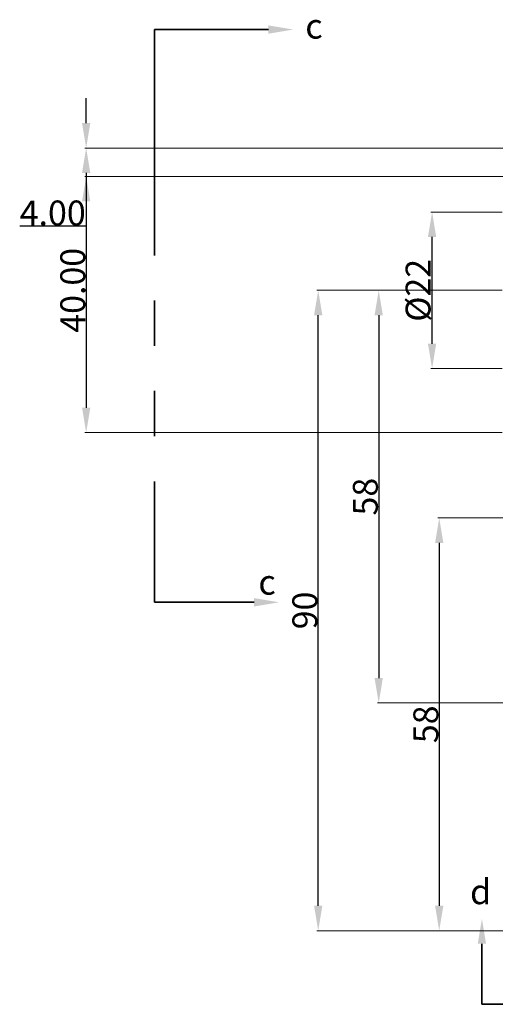
# Model space of a CAD drawing. Units: millimetres. Extents: x 75 to 489, y 21 to 350.
# Tile 2 of 5: x 75 to 142, y 199 to 337. Entities that reach past the tile are written whole.
import ezdxf

# ---------------------------------------------------------------- set-up
doc = ezdxf.new("R2010")
doc.units = ezdxf.units.MM
doc.header["$MEASUREMENT"] = 0
doc.linetypes.add('PHANTOM', pattern=[63.5, 31.75, -6.35, 6.35, -6.35, 6.35, -6.35])
for name, color, linetype, lineweight in [('M-DIMS', 2, 'Continuous', 25), ('M-SECT', 3, 'PHANTOM', 35), ('M-TEXT', 7, 'Continuous', 25)]:
    doc.layers.add(name, color=color, linetype=linetype, lineweight=lineweight)
doc.styles.get("Standard").update_dxf_attribs({"font": 'arial.ttf'})
doc.dimstyles.get("Standard").update_dxf_attribs({"dimtxt": 3.5, "dimasz": 3.5, "dimexe": 0.18, "dimexo": 0.0625, "dimgap": 0.09, "dimtad": 1, "dimtoh": 1, "dimdec": 0, "dimzin": 0, "dimdsep": 46, "dimtxsty": 'Standard', "dimcen": 0.09, "dimclrd": 2, "dimclre": 251, "dimadec": 0, "dimazin": 0, "dimtfac": 1, "dimtdec": 0, "dimtofl": 0, "dimtmove": 0, "dimatfit": 3, "dimfxl": 1, "dimtolj": 1, "dimtzin": 0, "dimlwe": 5, "dimarcsym": 0})

# ---------------------------------------------------------------- blocks, each defined once
blk = doc.blocks.new('*D24')
at = {"layer": 'Defpoints', "color": 0, "transparency": 16777216}
for p in [(133, 310.35), (142.9, 310.35), (142.9, 288.35)]:
    blk.add_point(p, dxfattribs=at)
at = {"layer": 'M-DIMS', "color": 0, "lineweight": 5, "transparency": 16777216}
for p, q in [((142.84, 310.35), (132.82, 310.35)), ((142.84, 288.35), (132.82, 288.35))]:
    blk.add_line(p, q, dxfattribs=at)
at = {"layer": 'M-DIMS', "color": 0, "lineweight": -2, "transparency": 16777216}
blk.add_line((133, 291.85), (133, 306.85), dxfattribs=at)
at = {"layer": 'M-DIMS', "color": 0, "transparency": 16777216}
for points in [[(132.42, 306.85), (133.58, 306.85), (133, 310.35)], [(132.42, 291.85), (133.58, 291.85), (133, 288.35)]]:
    blk.add_solid(points, dxfattribs=at)
at = {"layer": 'M-DIMS', "color": 0, "transparency": 16777216, "insert": (131.03, 299.35), "char_height": 3.5, "attachment_point": 5, "rotation": 90}
blk.add_mtext('\\A1;%%C22', dxfattribs=at)
blk = doc.blocks.new('*D25')
at = {"layer": 'Defpoints', "color": 0, "transparency": 16777216}
for p in [(142.9, 299.35), (125.5, 241.35), (232.9, 241.35)]:
    blk.add_point(p, dxfattribs=at)
at = {"layer": 'M-DIMS', "color": 0, "lineweight": 5, "transparency": 16777216}
for p, q in [((142.84, 299.35), (125.32, 299.35)), ((232.84, 241.35), (125.32, 241.35))]:
    blk.add_line(p, q, dxfattribs=at)
at = {"layer": 'M-DIMS', "color": 0, "lineweight": -2, "transparency": 16777216}
blk.add_line((125.5, 295.85), (125.5, 244.85), dxfattribs=at)
at = {"layer": 'M-DIMS', "color": 0, "transparency": 16777216}
for points in [[(124.92, 295.85), (126.08, 295.85), (125.5, 299.35)], [(124.92, 244.85), (126.08, 244.85), (125.5, 241.35)]]:
    blk.add_solid(points, dxfattribs=at)
at = {"layer": 'M-DIMS', "color": 0, "transparency": 16777216, "insert": (123.62, 270.35), "char_height": 3.5, "attachment_point": 5, "rotation": 90}
blk.add_mtext('\\A1;58', dxfattribs=at)
blk = doc.blocks.new('*D26')
at = {"layer": 'Defpoints', "color": 0, "transparency": 16777216}
for p in [(117, 299.35), (142.9, 299.35), (155.4, 209.35)]:
    blk.add_point(p, dxfattribs=at)
at = {"layer": 'M-DIMS', "color": 0, "lineweight": 5, "transparency": 16777216}
for p, q in [((142.84, 299.35), (116.82, 299.35)), ((155.34, 209.35), (116.82, 209.35))]:
    blk.add_line(p, q, dxfattribs=at)
at = {"layer": 'M-DIMS', "color": 0, "lineweight": -2, "transparency": 16777216}
blk.add_line((117, 212.85), (117, 295.85), dxfattribs=at)
at = {"layer": 'M-DIMS', "color": 0, "transparency": 16777216}
for points in [[(116.42, 295.85), (117.58, 295.85), (117, 299.35)], [(116.42, 212.85), (117.58, 212.85), (117, 209.35)]]:
    blk.add_solid(points, dxfattribs=at)
at = {"layer": 'M-DIMS', "color": 0, "transparency": 16777216, "insert": (115.12, 254.35), "char_height": 3.5, "attachment_point": 5, "rotation": 90}
blk.add_mtext('\\A1;90', dxfattribs=at)
blk = doc.blocks.new('*D27')
at = {"layer": 'Defpoints', "color": 0, "transparency": 16777216}
for p in [(171.9, 267.35), (134, 209.35), (155.4, 209.35)]:
    blk.add_point(p, dxfattribs=at)
at = {"layer": 'M-DIMS', "color": 0, "lineweight": 5, "transparency": 16777216}
for p, q in [((171.84, 267.35), (133.82, 267.35)), ((155.34, 209.35), (133.82, 209.35))]:
    blk.add_line(p, q, dxfattribs=at)
at = {"layer": 'M-DIMS', "color": 0, "lineweight": -2, "transparency": 16777216}
blk.add_line((134, 263.85), (134, 212.85), dxfattribs=at)
at = {"layer": 'M-DIMS', "color": 0, "transparency": 16777216}
for points in [[(133.42, 263.85), (134.58, 263.85), (134, 267.35)], [(133.42, 212.85), (134.58, 212.85), (134, 209.35)]]:
    blk.add_solid(points, dxfattribs=at)
at = {"layer": 'M-DIMS', "color": 0, "transparency": 16777216, "insert": (132.12, 238.35), "char_height": 3.5, "attachment_point": 5, "rotation": 90}
blk.add_mtext('\\A1;58', dxfattribs=at)
blk = doc.blocks.new('*D49')
at = {"layer": 'Defpoints', "color": 0, "transparency": 16777216}
for p in [(142.9, 319.35), (84.4, 279.35), (142.9, 279.35)]:
    blk.add_point(p, dxfattribs=at)
at = {"layer": 'M-DIMS', "color": 251, "lineweight": 5, "transparency": 16777216}
for p, q in [((142.84, 319.35), (84.22, 319.35)), ((142.84, 279.35), (84.22, 279.35))]:
    blk.add_line(p, q, dxfattribs=at)
at = {"layer": 'M-DIMS', "color": 2, "lineweight": -2, "transparency": 16777216}
blk.add_line((84.4, 315.85), (84.4, 282.85), dxfattribs=at)
at = {"layer": 'M-DIMS', "color": 2, "transparency": 16777216}
for points in [[(83.82, 315.85), (84.98, 315.85), (84.4, 319.35)], [(83.82, 282.85), (84.98, 282.85), (84.4, 279.35)]]:
    blk.add_solid(points, dxfattribs=at)
at = {"layer": 'M-DIMS', "color": 0, "transparency": 16777216, "insert": (82.52, 299.35), "char_height": 3.5, "attachment_point": 5, "rotation": 90}
blk.add_mtext('\\A1;40.00', dxfattribs=at)
blk = doc.blocks.new('*D60')
at = {"layer": 'Defpoints', "color": 0, "transparency": 16777216}
for p in [(152.9, 319.35), (84.4, 315.35), (152.9, 315.35)]:
    blk.add_point(p, dxfattribs=at)
at = {"layer": 'M-DIMS', "color": 2, "lineweight": -2, "transparency": 16777216}
for p, q in [((84.4, 322.85), (84.4, 326.35)), ((84.4, 311.85), (84.4, 308.35)), ((84.4, 308.35), (75.09, 308.35))]:
    blk.add_line(p, q, dxfattribs=at)
at = {"layer": 'M-DIMS', "color": 251, "lineweight": 5, "transparency": 16777216}
for p, q in [((152.84, 319.35), (84.22, 319.35)), ((152.84, 315.35), (84.22, 315.35))]:
    blk.add_line(p, q, dxfattribs=at)
at = {"layer": 'M-DIMS', "color": 2, "transparency": 16777216}
for points in [[(83.82, 322.85), (84.98, 322.85), (84.4, 319.35)], [(83.82, 311.85), (84.98, 311.85), (84.4, 315.35)]]:
    blk.add_solid(points, dxfattribs=at)
at = {"layer": 'M-DIMS', "color": 0, "transparency": 16777216, "insert": (79.7, 310.22), "char_height": 3.5, "attachment_point": 5}
blk.add_mtext('\\A1;4.00', dxfattribs=at)

msp = doc.modelspace()

# ---------------------------------------------------------------- linework, layer by layer
at = {"layer": 'M-SECT'}
for points in [[(110, 336), (94, 336), (94, 255.5)], [(108, 255.5), (94, 255.5)], [(140, 207.5), (140, 199), (191, 199)]]:
    msp.add_lwpolyline(points, dxfattribs=at)
for points in [[(110, 336.583), (113.5, 336), (110, 335.417)], [(108, 256.083), (111.5, 255.5), (108, 254.917)], [(139.417, 207.5), (140, 211), (140.583, 207.5)]]:
    msp.add_solid(points, dxfattribs=at)

# ---------------------------------------------------------------- texts
at = {"layer": 'M-TEXT', "char_height": 3.5, "attachment_point": 5}
for s, insert in [('\\A1;c', (116.404, 336.475)), ('\\A1;c', (109.814, 258.323)), ('\\A1;d', (139.814, 214.823))]:
    msp.add_mtext(s, dxfattribs=dict(at, insert=insert))

# ---------------------------------------------------------------- dimensions: what is measured, and where the dimension line sits
at = {"layer": 'M-DIMS'}
for base, p1, p2, override, picture, middle in [((84.4, 315.347), (152.904, 319.347), (152.904, 315.347), {"dimdec": 2, "dimlfac": 1, "dimrnd": 0, "dimzin": 0, "dimdsep": 46, "dimlunit": 2}, '*D60', (79.7, 310.224)), ((84.4, 279.347), (142.904, 319.347), (142.904, 279.347), {"dimdec": 2, "dimlfac": 1, "dimrnd": 0, "dimzin": 0, "dimdsep": 46, "dimlunit": 2}, '*D49', (82.523, 299.347)), ((117, 299.347), (155.404, 209.347), (142.904, 299.347), {"dimclrd": 0, "dimclre": 0, "dimclrt": 0}, '*D26', (115.123, 254.347)), ((125.5, 241.347), (142.904, 299.347), (232.904, 241.347), {"dimclrd": 0, "dimclre": 0, "dimclrt": 0}, '*D25', (123.623, 270.347)), ((134, 209.347), (171.904, 267.347), (155.404, 209.347), {"dimclrd": 0, "dimclre": 0, "dimclrt": 0}, '*D27', (132.123, 238.347))]:
    dim = msp.add_linear_dim(base=base, p1=p1, p2=p2, angle=90, dimstyle='Standard', override=override, dxfattribs=at)
    dim.commit()
    dim.dimension.update_dxf_attribs({"geometry": picture, "text_midpoint": middle})
dim = msp.add_linear_dim(base=(133, 310.347), p1=(142.904, 288.347), p2=(142.904, 310.347), angle=90, text='%%C<>', dimstyle='Standard', override={"dimclrd": 0, "dimclre": 0, "dimclrt": 0}, dxfattribs=at)
dim.commit()
dim.dimension.update_dxf_attribs({"geometry": '*D24', "text_midpoint": (131.025, 299.347)})

doc.saveas('drawing.dxf')
